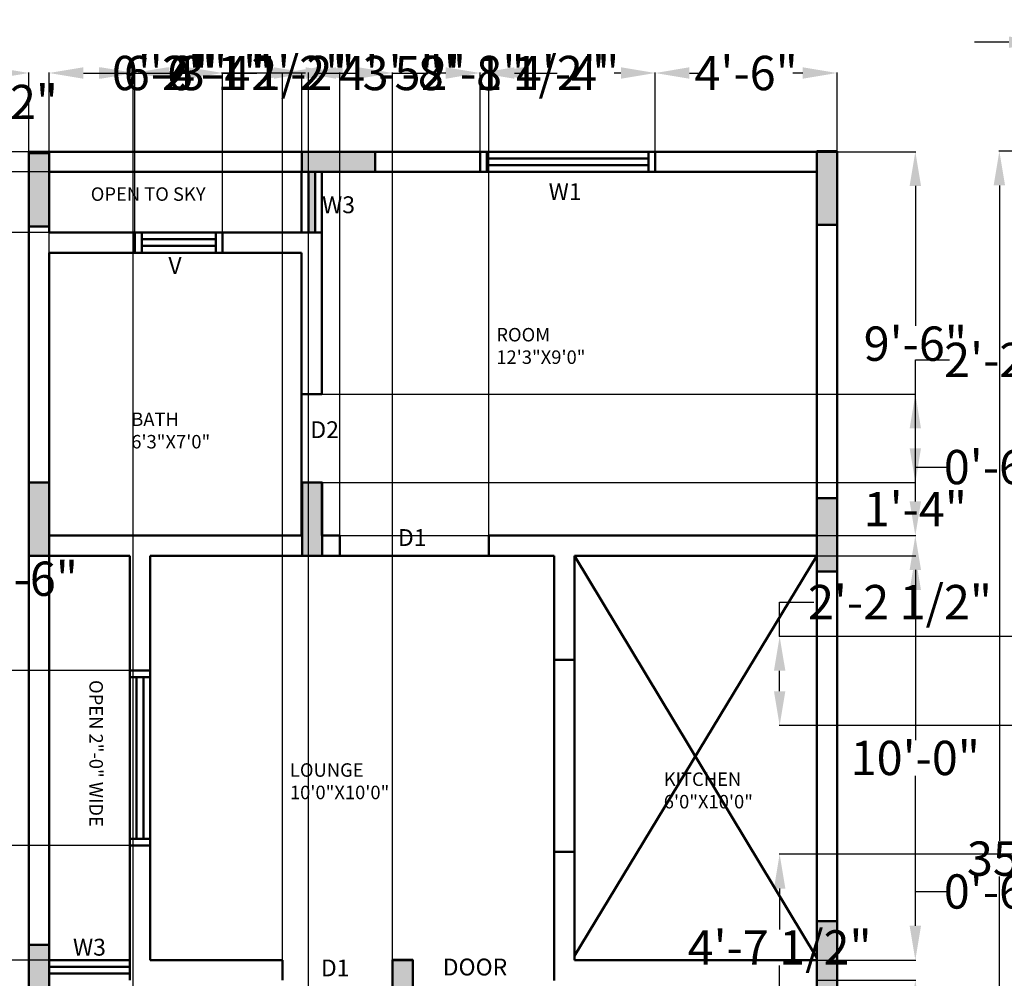
# Model space of a CAD drawing. Units: inches. Extents: x 21 to 3450, y 4 to 2137.
# Tile 4 of 14: x 2513 to 2805, y 1261 to 1546. Entities that reach past the tile are written whole.
import ezdxf

# ---------------------------------------------------------------- set-up
doc = ezdxf.new("R2010")
doc.units = ezdxf.units.IN
doc.header["$MEASUREMENT"] = 0
for name, color, linetype, lineweight in [('A-ANNO-DIMS', 2, 'Continuous', 18), ('A-ANNO-TEXT', 7, 'Continuous', 18), ('A-AREA-IDEN', 3, 'Continuous', 18), ('A-WALL', 7, 'Continuous', 50), ('A-WALL-PATT', 8, 'Continuous', 13)]:
    doc.layers.add(name, color=color, linetype=linetype, lineweight=lineweight)
doc.styles.get("Standard").update_dxf_attribs({"font": 'arial.ttf'})
doc.dimstyles.get("Standard").update_dxf_attribs({"dimtxt": 10.18, "dimasz": 10.18, "dimexe": 0.18, "dimexo": 0.0625, "dimgap": 0.09, "dimtad": 0, "dimtih": 1, "dimtoh": 1, "dimdec": 0, "dimzin": 0, "dimdsep": 46, "dimlunit": 3, "dimtxsty": 'Standard', "dimcen": 0.09, "dimadec": 0, "dimazin": 0, "dimtfac": 1, "dimtdec": 0, "dimtofl": 0, "dimtmove": 0, "dimatfit": 3, "dimfxl": 1, "dimtolj": 1, "dimtzin": 0, "dimarcsym": 0})

# ---------------------------------------------------------------- blocks, each defined once
blk = doc.blocks.new('*D8')
at = {"layer": 'A-ANNO-DIMS', "color": 0, "lineweight": -2, "transparency": 16777216}
for p, q in [((2816.85, 1506.81), (2803.73, 1506.81)), ((2803.91, 1496.63), (2803.91, 1302.07)), ((2803.91, 1096.92), (2803.91, 1291.48)), ((2999.5, 1086.74), (2803.73, 1086.74))]:
    blk.add_line(p, q, dxfattribs=at)
at = {"layer": 'A-ANNO-DIMS', "color": 0, "transparency": 16777216}
for points in [[(2802.22, 1496.63), (2805.61, 1496.63), (2803.91, 1506.81)], [(2802.22, 1096.92), (2805.61, 1096.92), (2803.91, 1086.74)]]:
    blk.add_solid(points, dxfattribs=at)
at = {"layer": 'Defpoints', "color": 0, "transparency": 16777216}
for p in [(2816.91, 1506.81), (2803.91, 1086.74), (2999.56, 1086.74)]:
    blk.add_point(p, dxfattribs=at)
at = {"layer": 'A-ANNO-DIMS', "color": 0, "transparency": 16777216, "insert": (2803.91, 1296.77), "char_height": 10.18, "attachment_point": 5}
blk.add_mtext("\\A1;35'", dxfattribs=at)
blk = doc.blocks.new('*D48')
at = {"layer": 'A-ANNO-DIMS', "color": 0, "lineweight": -2, "transparency": 16777216}
for p, q in [((2491.15, 1369.68), (2491.15, 1379.86)), ((2491.15, 1379.86), (2501.33, 1379.86)), ((2461.46, 1359.5), (2491.33, 1359.5)), ((2461.25, 1353.55), (2491.33, 1353.55)), ((2491.15, 1343.37), (2491.15, 1333.19))]:
    blk.add_line(p, q, dxfattribs=at)
at = {"layer": 'A-ANNO-DIMS', "color": 0, "transparency": 16777216}
for points in [[(2489.45, 1369.68), (2492.84, 1369.68), (2491.15, 1359.5)], [(2489.45, 1343.37), (2492.84, 1343.37), (2491.15, 1353.55)]]:
    blk.add_solid(points, dxfattribs=at)
at = {"layer": 'Defpoints', "color": 0, "transparency": 16777216}
for p in [(2461.4, 1359.5), (2491.15, 1359.5), (2461.19, 1353.55)]:
    blk.add_point(p, dxfattribs=at)
at = {"layer": 'A-ANNO-DIMS', "color": 0, "transparency": 16777216, "insert": (2514.95, 1379.86), "char_height": 10.18, "attachment_point": 5}
blk.add_mtext('\\A1;0\'-6"', dxfattribs=at)
blk = doc.blocks.new('*D63')
at = {"layer": 'A-ANNO-DIMS', "color": 0, "lineweight": -2, "transparency": 16777216}
for p, q in [((2417.71, 1189.56), (2417.71, 1521.59)), ((2427.89, 1521.41), (2451.22, 1521.41)), ((2461.4, 1189.56), (2461.4, 1521.59)), ((2461.4, 1521.41), (2471.58, 1521.41))]:
    blk.add_line(p, q, dxfattribs=at)
at = {"layer": 'A-ANNO-DIMS', "color": 0, "transparency": 16777216}
for points in [[(2427.89, 1523.11), (2427.89, 1519.72), (2417.71, 1521.41)], [(2451.22, 1523.11), (2451.22, 1519.72), (2461.4, 1521.41)]]:
    blk.add_solid(points, dxfattribs=at)
at = {"layer": 'Defpoints', "color": 0, "transparency": 16777216}
for p in [(2461.4, 1521.41), (2417.71, 1189.5), (2461.4, 1189.5)]:
    blk.add_point(p, dxfattribs=at)
at = {"layer": 'A-ANNO-DIMS', "color": 0, "transparency": 16777216, "insert": (2497.05, 1521.41), "char_height": 10.18, "attachment_point": 5}
blk.add_mtext('\\A1;3\'-7 1/2"', dxfattribs=at)
blk = doc.blocks.new('*D67')
at = {"layer": 'A-ANNO-DIMS', "color": 0, "lineweight": -2, "transparency": 16777216}
for p, q in [((2515.64, 1506.65), (2492.19, 1506.65)), ((2492.37, 1496.47), (2492.37, 1301.94)), ((2492.37, 1096.83), (2492.37, 1291.36)), ((2515.56, 1086.65), (2492.19, 1086.65))]:
    blk.add_line(p, q, dxfattribs=at)
at = {"layer": 'A-ANNO-DIMS', "color": 0, "transparency": 16777216}
for points in [[(2490.67, 1496.47), (2494.06, 1496.47), (2492.37, 1506.65)], [(2490.67, 1096.83), (2494.06, 1096.83), (2492.37, 1086.65)]]:
    blk.add_solid(points, dxfattribs=at)
at = {"layer": 'Defpoints', "color": 0, "transparency": 16777216}
for p in [(2492.37, 1506.65), (2515.71, 1506.65), (2515.62, 1086.65)]:
    blk.add_point(p, dxfattribs=at)
at = {"layer": 'A-ANNO-DIMS', "color": 0, "transparency": 16777216, "insert": (2492.37, 1296.65), "char_height": 10.18, "attachment_point": 5}
blk.add_mtext('\\A1;35\'-0"', dxfattribs=at)
blk = doc.blocks.new('*D68')
at = {"layer": 'A-ANNO-DIMS', "color": 0, "lineweight": -2, "transparency": 16777216}
for p, q in [((2505.53, 1530.01), (2495.35, 1530.01)), ((2515.71, 1506.71), (2515.71, 1530.19)), ((2521.71, 1500.71), (2521.71, 1530.19)), ((2531.89, 1530.01), (2542.07, 1530.01))]:
    blk.add_line(p, q, dxfattribs=at)
at = {"layer": 'A-ANNO-DIMS', "color": 0, "transparency": 16777216}
for points in [[(2505.53, 1531.71), (2505.53, 1528.31), (2515.71, 1530.01)], [(2531.89, 1531.71), (2531.89, 1528.31), (2521.71, 1530.01)]]:
    blk.add_solid(points, dxfattribs=at)
at = {"layer": 'Defpoints', "color": 0, "transparency": 16777216}
for p in [(2521.71, 1530.01), (2515.71, 1506.65), (2521.71, 1500.65)]:
    blk.add_point(p, dxfattribs=at)
at = {"layer": 'A-ANNO-DIMS', "color": 0, "transparency": 16777216, "insert": (2555.69, 1530.01), "char_height": 10.18, "attachment_point": 5}
blk.add_mtext('\\A1;0\'-6"', dxfattribs=at)
blk = doc.blocks.new('*D69')
at = {"layer": 'A-ANNO-DIMS', "color": 0, "lineweight": -2, "transparency": 16777216}
for p, q in [((2521.71, 1500.71), (2521.71, 1530.19)), ((2531.89, 1530.01), (2545.6, 1530.01)), ((2586.6, 1530.01), (2572.89, 1530.01)), ((2596.78, 1500.71), (2596.78, 1530.19))]:
    blk.add_line(p, q, dxfattribs=at)
at = {"layer": 'A-ANNO-DIMS', "color": 0, "transparency": 16777216}
for points in [[(2531.89, 1531.71), (2531.89, 1528.31), (2521.71, 1530.01)], [(2586.6, 1531.71), (2586.6, 1528.31), (2596.78, 1530.01)]]:
    blk.add_solid(points, dxfattribs=at)
at = {"layer": 'Defpoints', "color": 0, "transparency": 16777216}
for p in [(2596.78, 1530.01), (2521.71, 1500.65), (2596.78, 1500.65)]:
    blk.add_point(p, dxfattribs=at)
at = {"layer": 'A-ANNO-DIMS', "color": 0, "transparency": 16777216, "insert": (2559.24, 1530.01), "char_height": 10.18, "attachment_point": 5}
blk.add_mtext('\\A1;6\'-3"', dxfattribs=at)
blk = doc.blocks.new('*D70')
at = {"layer": 'A-ANNO-DIMS', "color": 0, "lineweight": -2, "transparency": 16777216}
for p, q in [((2596.78, 1500.71), (2596.78, 1530.19)), ((2606.96, 1530.01), (2609.42, 1530.01)), ((2639.52, 1530.01), (2637.07, 1530.01)), ((2649.7, 1506.71), (2649.7, 1530.19))]:
    blk.add_line(p, q, dxfattribs=at)
at = {"layer": 'A-ANNO-DIMS', "color": 0, "transparency": 16777216}
for points in [[(2606.96, 1531.71), (2606.96, 1528.31), (2596.78, 1530.01)], [(2639.52, 1531.71), (2639.52, 1528.31), (2649.7, 1530.01)]]:
    blk.add_solid(points, dxfattribs=at)
at = {"layer": 'Defpoints', "color": 0, "transparency": 16777216}
for p in [(2649.7, 1530.01), (2649.7, 1506.65), (2596.78, 1500.65)]:
    blk.add_point(p, dxfattribs=at)
at = {"layer": 'A-ANNO-DIMS', "color": 0, "transparency": 16777216, "insert": (2623.24, 1530.01), "char_height": 10.18, "attachment_point": 5}
blk.add_mtext('\\A1;4\'-5"', dxfattribs=at)
blk = doc.blocks.new('*D71')
at = {"layer": 'A-ANNO-DIMS', "color": 0, "lineweight": -2, "transparency": 16777216}
for p, q in [((2649.7, 1506.71), (2649.7, 1530.19)), ((2659.88, 1530.01), (2661.88, 1530.01)), ((2691.52, 1530.01), (2689.53, 1530.01)), ((2701.7, 1506.71), (2701.7, 1530.19))]:
    blk.add_line(p, q, dxfattribs=at)
at = {"layer": 'A-ANNO-DIMS', "color": 0, "transparency": 16777216}
for points in [[(2659.88, 1531.71), (2659.88, 1528.31), (2649.7, 1530.01)], [(2691.52, 1531.71), (2691.52, 1528.31), (2701.7, 1530.01)]]:
    blk.add_solid(points, dxfattribs=at)
at = {"layer": 'Defpoints', "color": 0, "transparency": 16777216}
for p in [(2701.7, 1530.01), (2649.7, 1506.65), (2701.7, 1506.65)]:
    blk.add_point(p, dxfattribs=at)
at = {"layer": 'A-ANNO-DIMS', "color": 0, "transparency": 16777216, "insert": (2675.7, 1530.01), "char_height": 10.18, "attachment_point": 5}
blk.add_mtext('\\A1;4\'-4"', dxfattribs=at)
blk = doc.blocks.new('*D72')
at = {"layer": 'A-ANNO-DIMS', "color": 0, "lineweight": -2, "transparency": 16777216}
for p, q in [((2701.7, 1506.71), (2701.7, 1530.19)), ((2711.88, 1530.01), (2714.88, 1530.01)), ((2745.53, 1530.01), (2742.53, 1530.01)), ((2755.71, 1506.71), (2755.71, 1530.19))]:
    blk.add_line(p, q, dxfattribs=at)
at = {"layer": 'A-ANNO-DIMS', "color": 0, "transparency": 16777216}
for points in [[(2711.88, 1531.71), (2711.88, 1528.31), (2701.7, 1530.01)], [(2745.53, 1531.71), (2745.53, 1528.31), (2755.71, 1530.01)]]:
    blk.add_solid(points, dxfattribs=at)
at = {"layer": 'Defpoints', "color": 0, "transparency": 16777216}
for p in [(2755.71, 1530.01), (2701.7, 1506.65), (2755.71, 1506.65)]:
    blk.add_point(p, dxfattribs=at)
at = {"layer": 'A-ANNO-DIMS', "color": 0, "transparency": 16777216, "insert": (2728.71, 1530.01), "char_height": 10.18, "attachment_point": 5}
blk.add_mtext('\\A1;4\'-6"', dxfattribs=at)
blk = doc.blocks.new('*D73')
at = {"layer": 'A-ANNO-DIMS', "color": 0, "lineweight": -2, "transparency": 16777216}
for p, q in [((2521.71, 1092.71), (2521.71, 1530.19)), ((2531.89, 1530.01), (2536.53, 1530.01)), ((2546.71, 1092.71), (2546.71, 1530.19)), ((2546.71, 1530.01), (2556.89, 1530.01))]:
    blk.add_line(p, q, dxfattribs=at)
at = {"layer": 'A-ANNO-DIMS', "color": 0, "transparency": 16777216}
for points in [[(2531.89, 1531.71), (2531.89, 1528.31), (2521.71, 1530.01)], [(2536.53, 1531.71), (2536.53, 1528.31), (2546.71, 1530.01)]]:
    blk.add_solid(points, dxfattribs=at)
at = {"layer": 'Defpoints', "color": 0, "transparency": 16777216}
for p in [(2546.71, 1530.01), (2521.71, 1092.65), (2546.71, 1092.65)]:
    blk.add_point(p, dxfattribs=at)
at = {"layer": 'A-ANNO-DIMS', "color": 0, "transparency": 16777216, "insert": (2570.59, 1530.01), "char_height": 10.18, "attachment_point": 5}
blk.add_mtext('\\A1;2\'-1"', dxfattribs=at)
blk = doc.blocks.new('*D74')
at = {"layer": 'A-ANNO-DIMS', "color": 0, "lineweight": -2, "transparency": 16777216}
for p, q in [((2546.71, 1092.71), (2546.71, 1530.19)), ((2556.89, 1530.01), (2558.88, 1530.01)), ((2588.53, 1530.01), (2586.53, 1530.01)), ((2598.71, 1092.71), (2598.71, 1530.19))]:
    blk.add_line(p, q, dxfattribs=at)
at = {"layer": 'A-ANNO-DIMS', "color": 0, "transparency": 16777216}
for points in [[(2556.89, 1531.71), (2556.89, 1528.31), (2546.71, 1530.01)], [(2588.53, 1531.71), (2588.53, 1528.31), (2598.71, 1530.01)]]:
    blk.add_solid(points, dxfattribs=at)
at = {"layer": 'Defpoints', "color": 0, "transparency": 16777216}
for p in [(2598.71, 1530.01), (2546.71, 1092.65), (2598.71, 1092.65)]:
    blk.add_point(p, dxfattribs=at)
at = {"layer": 'A-ANNO-DIMS', "color": 0, "transparency": 16777216, "insert": (2572.71, 1530.01), "char_height": 10.18, "attachment_point": 5}
blk.add_mtext('\\A1;4\'-4"', dxfattribs=at)
blk = doc.blocks.new('*D75')
at = {"layer": 'A-ANNO-DIMS', "color": 0, "lineweight": -2, "transparency": 16777216}
for p, q in [((2598.71, 1092.71), (2598.71, 1530.19)), ((2608.89, 1530.01), (2613.53, 1530.01)), ((2623.71, 1092.71), (2623.71, 1530.19)), ((2623.71, 1530.01), (2633.89, 1530.01))]:
    blk.add_line(p, q, dxfattribs=at)
at = {"layer": 'A-ANNO-DIMS', "color": 0, "transparency": 16777216}
for points in [[(2608.89, 1531.71), (2608.89, 1528.31), (2598.71, 1530.01)], [(2613.53, 1531.71), (2613.53, 1528.31), (2623.71, 1530.01)]]:
    blk.add_solid(points, dxfattribs=at)
at = {"layer": 'Defpoints', "color": 0, "transparency": 16777216}
for p in [(2623.71, 1530.01), (2598.71, 1092.65), (2623.71, 1092.65)]:
    blk.add_point(p, dxfattribs=at)
at = {"layer": 'A-ANNO-DIMS', "color": 0, "transparency": 16777216, "insert": (2647.59, 1530.01), "char_height": 10.18, "attachment_point": 5}
blk.add_mtext('\\A1;2\'-1"', dxfattribs=at)
blk = doc.blocks.new('*D77')
at = {"layer": 'A-ANNO-DIMS', "color": 0, "lineweight": -2, "transparency": 16777216}
for p, q in [((2778.96, 1276.83), (2778.96, 1287.01)), ((2778.96, 1287.01), (2789.14, 1287.01)), ((2749.77, 1266.65), (2779.14, 1266.65)), ((2749.77, 1260.65), (2779.14, 1260.65)), ((2778.96, 1250.47), (2778.96, 1240.29))]:
    blk.add_line(p, q, dxfattribs=at)
at = {"layer": 'A-ANNO-DIMS', "color": 0, "transparency": 16777216}
for points in [[(2777.26, 1276.83), (2780.65, 1276.83), (2778.96, 1266.65)], [(2777.26, 1250.47), (2780.65, 1250.47), (2778.96, 1260.65)]]:
    blk.add_solid(points, dxfattribs=at)
at = {"layer": 'Defpoints', "color": 0, "transparency": 16777216}
for p in [(2749.71, 1266.65), (2778.96, 1266.65), (2749.71, 1260.65)]:
    blk.add_point(p, dxfattribs=at)
at = {"layer": 'A-ANNO-DIMS', "color": 0, "transparency": 16777216, "insert": (2802.76, 1287.01), "char_height": 10.18, "attachment_point": 5}
blk.add_mtext('\\A1;0\'-6"', dxfattribs=at)
blk = doc.blocks.new('*D78')
at = {"layer": 'A-ANNO-DIMS', "color": 0, "lineweight": -2, "transparency": 16777216}
for p, q in [((2749.77, 1386.65), (2779.14, 1386.65)), ((2778.96, 1376.47), (2778.96, 1331.94)), ((2778.96, 1276.83), (2778.96, 1321.36)), ((2749.77, 1266.65), (2779.14, 1266.65))]:
    blk.add_line(p, q, dxfattribs=at)
at = {"layer": 'A-ANNO-DIMS', "color": 0, "transparency": 16777216}
for points in [[(2777.26, 1376.47), (2780.65, 1376.47), (2778.96, 1386.65)], [(2777.26, 1276.83), (2780.65, 1276.83), (2778.96, 1266.65)]]:
    blk.add_solid(points, dxfattribs=at)
at = {"layer": 'Defpoints', "color": 0, "transparency": 16777216}
for p in [(2749.71, 1386.65), (2778.96, 1386.65), (2749.71, 1266.65)]:
    blk.add_point(p, dxfattribs=at)
at = {"layer": 'A-ANNO-DIMS', "color": 0, "transparency": 16777216, "insert": (2778.96, 1326.65), "char_height": 10.18, "attachment_point": 5}
blk.add_mtext('\\A1;10\'-0"', dxfattribs=at)
blk = doc.blocks.new('*D79')
at = {"layer": 'A-ANNO-DIMS', "color": 0, "lineweight": -2, "transparency": 16777216}
for p, q in [((2778.96, 1402.83), (2778.96, 1413.01)), ((2778.96, 1413.01), (2789.14, 1413.01)), ((2749.77, 1392.65), (2779.14, 1392.65)), ((2749.77, 1386.65), (2779.14, 1386.65)), ((2778.96, 1376.47), (2778.96, 1366.29))]:
    blk.add_line(p, q, dxfattribs=at)
at = {"layer": 'A-ANNO-DIMS', "color": 0, "transparency": 16777216}
for points in [[(2777.26, 1402.83), (2780.65, 1402.83), (2778.96, 1392.65)], [(2777.26, 1376.47), (2780.65, 1376.47), (2778.96, 1386.65)]]:
    blk.add_solid(points, dxfattribs=at)
at = {"layer": 'Defpoints', "color": 0, "transparency": 16777216}
for p in [(2749.71, 1392.65), (2778.96, 1392.65), (2749.71, 1386.65)]:
    blk.add_point(p, dxfattribs=at)
at = {"layer": 'A-ANNO-DIMS', "color": 0, "transparency": 16777216, "insert": (2802.76, 1413.01), "char_height": 10.18, "attachment_point": 5}
blk.add_mtext('\\A1;0\'-6"', dxfattribs=at)
blk = doc.blocks.new('*D80')
at = {"layer": 'A-ANNO-DIMS', "color": 0, "lineweight": -2, "transparency": 16777216}
for p, q in [((2755.77, 1506.65), (2779.14, 1506.65)), ((2778.96, 1496.47), (2778.96, 1454.94)), ((2778.96, 1402.83), (2778.96, 1444.36)), ((2749.77, 1392.65), (2779.14, 1392.65))]:
    blk.add_line(p, q, dxfattribs=at)
at = {"layer": 'A-ANNO-DIMS', "color": 0, "transparency": 16777216}
for points in [[(2777.26, 1496.47), (2780.65, 1496.47), (2778.96, 1506.65)], [(2777.26, 1402.83), (2780.65, 1402.83), (2778.96, 1392.65)]]:
    blk.add_solid(points, dxfattribs=at)
at = {"layer": 'Defpoints', "color": 0, "transparency": 16777216}
for p in [(2755.71, 1506.65), (2778.96, 1506.65), (2749.71, 1392.65)]:
    blk.add_point(p, dxfattribs=at)
at = {"layer": 'A-ANNO-DIMS', "color": 0, "transparency": 16777216, "insert": (2778.96, 1449.65), "char_height": 10.18, "attachment_point": 5}
blk.add_mtext('\\A1;9\'-6"', dxfattribs=at)
blk = doc.blocks.new('*D81')
at = {"layer": 'A-ANNO-DIMS', "color": 0, "lineweight": -2, "transparency": 16777216}
for p, q in [((2492.37, 1510.83), (2492.37, 1521.01)), ((2521.64, 1500.65), (2492.19, 1500.65)), ((2521.64, 1482.65), (2492.19, 1482.65)), ((2492.37, 1472.47), (2492.37, 1462.29))]:
    blk.add_line(p, q, dxfattribs=at)
at = {"layer": 'A-ANNO-DIMS', "color": 0, "transparency": 16777216}
for points in [[(2490.67, 1510.83), (2494.06, 1510.83), (2492.37, 1500.65)], [(2490.67, 1472.47), (2494.06, 1472.47), (2492.37, 1482.65)]]:
    blk.add_solid(points, dxfattribs=at)
at = {"layer": 'Defpoints', "color": 0, "transparency": 16777216}
for p in [(2492.37, 1500.65), (2521.71, 1500.65), (2521.71, 1482.65)]:
    blk.add_point(p, dxfattribs=at)
at = {"layer": 'A-ANNO-DIMS', "color": 0, "transparency": 16777216, "insert": (2492.37, 1491.65), "char_height": 10.18, "attachment_point": 5}
blk.add_mtext('\\A1;1\'-6"', dxfattribs=at)
blk = doc.blocks.new('*D82')
at = {"layer": 'A-ANNO-DIMS', "color": 0, "lineweight": -2, "transparency": 16777216}
for p, q in [((2778.96, 1434.65), (2778.96, 1444.83)), ((2778.96, 1444.83), (2789.14, 1444.83)), ((2602.77, 1434.65), (2779.14, 1434.65)), ((2778.96, 1418.61), (2778.96, 1424.47)), ((2602.9, 1408.43), (2779.14, 1408.43))]:
    blk.add_line(p, q, dxfattribs=at)
at = {"layer": 'A-ANNO-DIMS', "color": 0, "transparency": 16777216}
for points in [[(2777.26, 1424.47), (2780.65, 1424.47), (2778.96, 1434.65)], [(2777.26, 1418.61), (2780.65, 1418.61), (2778.96, 1408.43)]]:
    blk.add_solid(points, dxfattribs=at)
at = {"layer": 'Defpoints', "color": 0, "transparency": 16777216}
for p in [(2602.71, 1434.65), (2778.96, 1434.65), (2602.84, 1408.43)]:
    blk.add_point(p, dxfattribs=at)
at = {"layer": 'A-ANNO-DIMS', "color": 0, "transparency": 16777216, "insert": (2802.84, 1444.83), "char_height": 10.18, "attachment_point": 5}
blk.add_mtext('\\A1;2\'-2"', dxfattribs=at)
blk = doc.blocks.new('*D83')
at = {"layer": 'A-ANNO-DIMS', "color": 0, "lineweight": -2, "transparency": 16777216}
for p, q in [((2778.96, 1418.61), (2778.96, 1428.79)), ((2602.9, 1408.43), (2779.14, 1408.43)), ((2602.77, 1392.65), (2779.14, 1392.65)), ((2778.96, 1382.47), (2778.96, 1372.29))]:
    blk.add_line(p, q, dxfattribs=at)
at = {"layer": 'A-ANNO-DIMS', "color": 0, "transparency": 16777216}
for points in [[(2777.26, 1418.61), (2780.65, 1418.61), (2778.96, 1408.43)], [(2777.26, 1382.47), (2780.65, 1382.47), (2778.96, 1392.65)]]:
    blk.add_solid(points, dxfattribs=at)
at = {"layer": 'Defpoints', "color": 0, "transparency": 16777216}
for p in [(2602.84, 1408.43), (2778.96, 1408.43), (2602.71, 1392.65)]:
    blk.add_point(p, dxfattribs=at)
at = {"layer": 'A-ANNO-DIMS', "color": 0, "transparency": 16777216, "insert": (2778.96, 1400.54), "char_height": 10.18, "attachment_point": 5}
blk.add_mtext('\\A1;1\'-4"', dxfattribs=at)
blk = doc.blocks.new('*D84')
at = {"layer": 'A-ANNO-DIMS', "color": 0, "lineweight": -2, "transparency": 16777216}
for p, q in [((2597.89, 1530.01), (2587.71, 1530.01)), ((2608.07, 1392.71), (2608.07, 1530.19)), ((2652.26, 1392.71), (2652.26, 1530.19)), ((2662.44, 1530.01), (2672.62, 1530.01))]:
    blk.add_line(p, q, dxfattribs=at)
at = {"layer": 'A-ANNO-DIMS', "color": 0, "transparency": 16777216}
for points in [[(2597.89, 1531.71), (2597.89, 1528.31), (2608.07, 1530.01)], [(2662.44, 1531.71), (2662.44, 1528.31), (2652.26, 1530.01)]]:
    blk.add_solid(points, dxfattribs=at)
at = {"layer": 'Defpoints', "color": 0, "transparency": 16777216}
for p in [(2652.26, 1530.01), (2608.07, 1392.65), (2652.26, 1392.65)]:
    blk.add_point(p, dxfattribs=at)
at = {"layer": 'A-ANNO-DIMS', "color": 0, "transparency": 16777216, "insert": (2630.16, 1530.01), "char_height": 10.18, "attachment_point": 5}
blk.add_mtext('\\A1;3\'-8"', dxfattribs=at)
blk = doc.blocks.new('*D85')
at = {"layer": 'A-ANNO-DIMS', "color": 0, "lineweight": -2, "transparency": 16777216}
for p, q in [((2591.07, 1266.71), (2591.07, 1530.19)), ((2601.25, 1530.01), (2613.53, 1530.01)), ((2623.71, 1266.71), (2623.71, 1530.19)), ((2623.71, 1530.01), (2633.89, 1530.01))]:
    blk.add_line(p, q, dxfattribs=at)
at = {"layer": 'A-ANNO-DIMS', "color": 0, "transparency": 16777216}
for points in [[(2601.25, 1531.71), (2601.25, 1528.31), (2591.07, 1530.01)], [(2613.53, 1531.71), (2613.53, 1528.31), (2623.71, 1530.01)]]:
    blk.add_solid(points, dxfattribs=at)
at = {"layer": 'Defpoints', "color": 0, "transparency": 16777216}
for p in [(2623.71, 1530.01), (2591.07, 1266.65), (2623.71, 1266.65)]:
    blk.add_point(p, dxfattribs=at)
at = {"layer": 'A-ANNO-DIMS', "color": 0, "transparency": 16777216, "insert": (2659.45, 1530.01), "char_height": 10.18, "attachment_point": 5}
blk.add_mtext('\\A1;2\'-8 1/2"', dxfattribs=at)
blk = doc.blocks.new('*D89')
at = {"layer": 'A-ANNO-DIMS', "color": 0, "lineweight": -2, "transparency": 16777216}
for p, q in [((2545.64, 1352.65), (2492.19, 1352.65)), ((2492.37, 1342.47), (2492.37, 1331.83)), ((2492.37, 1310.83), (2492.37, 1321.47)), ((2545.64, 1300.65), (2492.19, 1300.65))]:
    blk.add_line(p, q, dxfattribs=at)
at = {"layer": 'A-ANNO-DIMS', "color": 0, "transparency": 16777216}
for points in [[(2490.67, 1342.47), (2494.06, 1342.47), (2492.37, 1352.65)], [(2490.67, 1310.83), (2494.06, 1310.83), (2492.37, 1300.65)]]:
    blk.add_solid(points, dxfattribs=at)
at = {"layer": 'Defpoints', "color": 0, "transparency": 16777216}
for p in [(2492.37, 1352.65), (2545.71, 1352.65), (2545.71, 1300.65)]:
    blk.add_point(p, dxfattribs=at)
at = {"layer": 'A-ANNO-DIMS', "color": 0, "transparency": 16777216, "insert": (2492.37, 1326.65), "char_height": 10.18, "attachment_point": 5}
blk.add_mtext('\\A1;4\'-4"', dxfattribs=at)
blk = doc.blocks.new('*D90')
at = {"layer": 'A-ANNO-DIMS', "color": 0, "lineweight": -2, "transparency": 16777216}
for p, q in [((2545.64, 1300.65), (2492.19, 1300.65)), ((2492.37, 1290.47), (2492.37, 1288.94)), ((2492.37, 1276.83), (2492.37, 1278.36)), ((2545.64, 1266.65), (2492.19, 1266.65))]:
    blk.add_line(p, q, dxfattribs=at)
at = {"layer": 'A-ANNO-DIMS', "color": 0, "transparency": 16777216}
for points in [[(2490.67, 1290.47), (2494.06, 1290.47), (2492.37, 1300.65)], [(2490.67, 1276.83), (2494.06, 1276.83), (2492.37, 1266.65)]]:
    blk.add_solid(points, dxfattribs=at)
at = {"layer": 'Defpoints', "color": 0, "transparency": 16777216}
for p in [(2492.37, 1300.65), (2545.71, 1300.65), (2545.71, 1266.65)]:
    blk.add_point(p, dxfattribs=at)
at = {"layer": 'A-ANNO-DIMS', "color": 0, "transparency": 16777216, "insert": (2492.37, 1283.65), "char_height": 10.18, "attachment_point": 5}
blk.add_mtext('\\A1;2\'-10"', dxfattribs=at)
blk = doc.blocks.new('*D91')
at = {"layer": 'A-ANNO-DIMS', "color": 0, "lineweight": -2, "transparency": 16777216}
for p, q in [((2521.71, 1476.71), (2521.71, 1530.19)), ((2531.89, 1530.01), (2537.03, 1530.01)), ((2547.21, 1476.71), (2547.21, 1530.19)), ((2547.21, 1530.01), (2557.39, 1530.01))]:
    blk.add_line(p, q, dxfattribs=at)
at = {"layer": 'A-ANNO-DIMS', "color": 0, "transparency": 16777216}
for points in [[(2531.89, 1531.71), (2531.89, 1528.31), (2521.71, 1530.01)], [(2537.03, 1531.71), (2537.03, 1528.31), (2547.21, 1530.01)]]:
    blk.add_solid(points, dxfattribs=at)
at = {"layer": 'Defpoints', "color": 0, "transparency": 16777216}
for p in [(2547.21, 1530.01), (2521.71, 1476.65), (2547.21, 1476.65)]:
    blk.add_point(p, dxfattribs=at)
at = {"layer": 'A-ANNO-DIMS', "color": 0, "transparency": 16777216, "insert": (2582.95, 1530.01), "char_height": 10.18, "attachment_point": 5}
blk.add_mtext('\\A1;2\'-1 1/2"', dxfattribs=at)
blk = doc.blocks.new('*D92')
at = {"layer": 'A-ANNO-DIMS', "color": 0, "lineweight": -2, "transparency": 16777216}
for p, q in [((2547.21, 1476.71), (2547.21, 1530.19)), ((2557.39, 1530.01), (2563.03, 1530.01)), ((2573.21, 1476.71), (2573.21, 1530.19)), ((2573.21, 1530.01), (2583.39, 1530.01))]:
    blk.add_line(p, q, dxfattribs=at)
at = {"layer": 'A-ANNO-DIMS', "color": 0, "transparency": 16777216}
for points in [[(2557.39, 1531.71), (2557.39, 1528.31), (2547.21, 1530.01)], [(2563.03, 1531.71), (2563.03, 1528.31), (2573.21, 1530.01)]]:
    blk.add_solid(points, dxfattribs=at)
at = {"layer": 'Defpoints', "color": 0, "transparency": 16777216}
for p in [(2573.21, 1530.01), (2547.21, 1476.65), (2573.21, 1476.65)]:
    blk.add_point(p, dxfattribs=at)
at = {"layer": 'A-ANNO-DIMS', "color": 0, "transparency": 16777216, "insert": (2597.09, 1530.01), "char_height": 10.18, "attachment_point": 5}
blk.add_mtext('\\A1;2\'-2"', dxfattribs=at)
blk = doc.blocks.new('*D96')
at = {"layer": 'A-ANNO-DIMS', "color": 0, "lineweight": -2, "transparency": 16777216}
for p, q in [((2806.73, 1539.16), (2796.55, 1539.16)), ((2816.91, 1506.81), (2816.91, 1539.34)), ((2822.91, 1500.81), (2822.91, 1539.34)), ((2833.09, 1539.16), (2843.27, 1539.16))]:
    blk.add_line(p, q, dxfattribs=at)
at = {"layer": 'A-ANNO-DIMS', "color": 0, "transparency": 16777216}
for points in [[(2806.73, 1540.85), (2806.73, 1537.46), (2816.91, 1539.16)], [(2833.09, 1540.85), (2833.09, 1537.46), (2822.91, 1539.16)]]:
    blk.add_solid(points, dxfattribs=at)
at = {"layer": 'Defpoints', "color": 0, "transparency": 16777216}
for p in [(2822.91, 1539.16), (2816.91, 1506.74), (2822.91, 1500.74)]:
    blk.add_point(p, dxfattribs=at)
at = {"layer": 'A-ANNO-DIMS', "color": 0, "transparency": 16777216, "insert": (2856.89, 1539.16), "char_height": 10.18, "attachment_point": 5}
blk.add_mtext('\\A1;0\'-6"', dxfattribs=at)
blk = doc.blocks.new('*D119')
at = {"layer": 'A-ANNO-DIMS', "color": 0, "lineweight": -2, "transparency": 16777216}
for p, q in [((2738.66, 1362.74), (2738.66, 1372.92)), ((2738.66, 1372.92), (2748.84, 1372.92)), ((2972.85, 1362.74), (2738.48, 1362.74)), ((2738.66, 1346.47), (2738.66, 1352.56)), ((2972.85, 1336.29), (2738.48, 1336.29))]:
    blk.add_line(p, q, dxfattribs=at)
at = {"layer": 'A-ANNO-DIMS', "color": 0, "transparency": 16777216}
for points in [[(2736.97, 1352.56), (2740.36, 1352.56), (2738.66, 1362.74)], [(2736.97, 1346.47), (2740.36, 1346.47), (2738.66, 1336.29)]]:
    blk.add_solid(points, dxfattribs=at)
at = {"layer": 'Defpoints', "color": 0, "transparency": 16777216}
for p in [(2738.66, 1362.74), (2972.91, 1362.74), (2972.91, 1336.29)]:
    blk.add_point(p, dxfattribs=at)
at = {"layer": 'A-ANNO-DIMS', "color": 0, "transparency": 16777216, "insert": (2774.41, 1372.92), "char_height": 10.18, "attachment_point": 5}
blk.add_mtext('\\A1;2\'-2 1/2"', dxfattribs=at)
blk = doc.blocks.new('*D120')
at = {"layer": 'A-ANNO-DIMS', "color": 0, "lineweight": -2, "transparency": 16777216}
for p, q in [((2972.85, 1298.07), (2738.48, 1298.07)), ((2738.66, 1287.89), (2738.66, 1275.76)), ((2738.66, 1252.92), (2738.66, 1265.05)), ((2972.85, 1242.74), (2738.48, 1242.74))]:
    blk.add_line(p, q, dxfattribs=at)
at = {"layer": 'A-ANNO-DIMS', "color": 0, "transparency": 16777216}
for points in [[(2736.97, 1287.89), (2740.36, 1287.89), (2738.66, 1298.07)], [(2736.97, 1252.92), (2740.36, 1252.92), (2738.66, 1242.74)]]:
    blk.add_solid(points, dxfattribs=at)
at = {"layer": 'Defpoints', "color": 0, "transparency": 16777216}
for p in [(2738.66, 1298.07), (2972.91, 1298.07), (2972.91, 1242.74)]:
    blk.add_point(p, dxfattribs=at)
at = {"layer": 'A-ANNO-DIMS', "color": 0, "transparency": 16777216, "insert": (2738.66, 1270.41), "char_height": 10.18, "attachment_point": 5}
blk.add_mtext('\\A1;4\'-7 1/2"', dxfattribs=at)

msp = doc.modelspace()

# ---------------------------------------------------------------- hatches: boundary and pattern name
at = {"layer": 'A-WALL-PATT'}
h = msp.add_hatch(color=256, dxfattribs=at)
h.dxf.hatch_style = 1
h.paths.add_polyline_path([(2521.71, 1506.22), (2515.71, 1506.22), (2515.71, 1484.44), (2521.71, 1484.44)])
h.paths.add_polyline_path([(2618.57, 1506.65), (2596.78, 1506.65), (2596.78, 1500.65), (2618.57, 1500.65)])
h.paths.add_polyline_path([(2755.71, 1506.65), (2749.71, 1506.65), (2749.71, 1484.98), (2755.71, 1484.98)])
h.paths.add_polyline_path([(2755.71, 1403.77), (2749.71, 1403.77), (2749.71, 1381.98), (2755.71, 1381.98)])
h.paths.add_polyline_path([(2602.71, 1408.43), (2596.84, 1408.43), (2596.84, 1386.65), (2602.84, 1386.65), (2602.84, 1392.65), (2602.71, 1392.65)])
h.paths.add_polyline_path([(2755.71, 1278.18), (2749.71, 1278.18), (2749.71, 1256.4), (2755.71, 1256.4)])
h.paths.add_polyline_path([(2521.71, 1271.12), (2515.71, 1271.12), (2515.71, 1249.33), (2521.71, 1249.33)])
h.paths.add_polyline_path([(2521.71, 1408.43), (2515.71, 1408.43), (2515.71, 1386.65), (2521.71, 1386.65)])
h.paths.add_polyline_path([(2629.71, 1266.65), (2623.71, 1266.65), (2623.71, 1244.92), (2629.71, 1244.92)])
h.paths.add_polyline_path([(2521.62, 1108.43), (2515.71, 1108.43), (2515.71, 1086.65), (2521.62, 1086.65)])
h.paths.add_polyline_path([(2629.43, 1108.43), (2623.71, 1108.43), (2623.71, 1092.65), (2623.43, 1086.65), (2629.43, 1086.65)])
h.paths.add_polyline_path([(2755.71, 1108.43), (2749.71, 1108.43), (2749.71, 1086.65), (2755.71, 1086.65)])
h = msp.add_hatch(color=256, dxfattribs=at)
h.dxf.hatch_style = 1
h.paths.add_polyline_path([(2600.71, 1500.65), (2598.71, 1500.65), (2598.71, 1482.65), (2600.71, 1482.65)])

# ---------------------------------------------------------------- linework, layer by layer
at = {"layer": 'A-WALL'}
for p, q in [((2515.71, 1086.65), (2515.71, 1506.65)), ((2515.71, 1506.65), (2755.71, 1506.65)), ((2649.7, 1500.65), (2649.7, 1506.65)), ((2651.7, 1500.65), (2651.7, 1506.65)), ((2699.7, 1500.65), (2699.7, 1506.65)), ((2701.7, 1500.65), (2701.7, 1506.65)), ((2755.71, 1506.65), (2755.71, 1086.65)), ((2651.7, 1504.65), (2699.7, 1504.65)), ((2521.71, 1500.65), (2749.71, 1500.65)), ((2521.71, 1482.65), (2521.71, 1500.65)), ((2596.71, 1500.65), (2596.71, 1482.65)), ((2598.71, 1482.65), (2598.71, 1500.65)), ((2600.71, 1482.65), (2600.71, 1500.65)), ((2602.71, 1500.65), (2602.71, 1434.65)), ((2651.7, 1502.65), (2699.7, 1502.65)), ((2749.71, 1500.65), (2749.71, 1392.65)), ((2521.71, 1482.65), (2596.71, 1482.65)), ((2547.21, 1482.65), (2547.21, 1476.65)), ((2549.21, 1482.65), (2549.21, 1476.65)), ((2571.21, 1482.65), (2571.21, 1476.65)), ((2573.21, 1482.65), (2573.21, 1476.65)), ((2596.71, 1482.65), (2602.71, 1482.65)), ((2549.21, 1480.65), (2571.21, 1480.65)), ((2521.71, 1476.65), (2596.71, 1476.65)), ((2521.71, 1392.65), (2521.71, 1476.65)), ((2549.21, 1478.65), (2571.21, 1478.65)), ((2596.71, 1476.65), (2596.71, 1392.65)), ((2596.71, 1434.65), (2602.71, 1434.65)), ((2602.71, 1408.43), (2602.71, 1392.65)), ((2521.71, 1392.65), (2596.71, 1392.65)), ((2602.71, 1392.65), (2608.07, 1392.65)), ((2608.07, 1392.65), (2608.07, 1386.65)), ((2652.26, 1386.65), (2652.26, 1392.65)), ((2652.26, 1392.65), (2749.71, 1392.65)), ((2521.71, 1386.65), (2545.71, 1386.65)), ((2521.71, 1266.65), (2521.71, 1386.65)), ((2545.71, 1386.65), (2545.71, 1266.65)), ((2551.71, 1386.65), (2551.71, 1266.65)), ((2551.71, 1386.65), (2671.71, 1386.65)), ((2671.71, 1386.65), (2671.71, 1266.65)), ((2677.71, 1386.65), (2677.71, 1266.65)), ((2677.71, 1386.65), (2749.71, 1386.65)), ((2677.71, 1386.65), (2749.71, 1267.29)), ((2749.71, 1386.65), (2677.71, 1267.94)), ((2749.71, 1386.65), (2749.71, 1266.65)), ((2671.71, 1355.74), (2677.71, 1355.74)), ((2551.71, 1352.65), (2545.71, 1352.65)), ((2551.71, 1350.65), (2545.71, 1350.65)), ((2547.71, 1350.65), (2547.71, 1302.65)), ((2549.71, 1350.65), (2549.71, 1302.65)), ((2549.71, 1350.65), (2549.71, 1302.65)), ((2551.71, 1302.65), (2545.71, 1302.65)), ((2551.71, 1300.65), (2545.71, 1300.65)), ((2671.71, 1298.78), (2677.71, 1298.78)), ((2521.71, 1266.65), (2545.71, 1266.65)), ((2521.71, 1266.65), (2521.71, 1260.65)), ((2545.71, 1266.65), (2545.71, 1260.65)), ((2551.71, 1266.65), (2591.07, 1266.65)), ((2591.07, 1266.65), (2591.07, 1260.65)), ((2623.71, 1266.65), (2629.71, 1266.65)), ((2671.71, 1266.65), (2671.71, 1260.57)), ((2677.71, 1266.65), (2749.71, 1266.65)), ((2545.71, 1264.65), (2521.71, 1264.65)), ((2545.71, 1262.65), (2521.71, 1262.65))]:
    msp.add_line(p, q, dxfattribs=at)
for points in [[(2515.71, 1506.22), (2521.71, 1506.22), (2521.71, 1484.44), (2515.71, 1484.44)], [(2596.78, 1500.65), (2596.78, 1506.65), (2618.57, 1506.65), (2618.57, 1500.65)], [(2749.71, 1506.76), (2755.71, 1506.76), (2755.71, 1484.98), (2749.71, 1484.98)], [(2515.71, 1408.43), (2521.71, 1408.43), (2521.71, 1386.65), (2515.71, 1386.65)], [(2596.84, 1408.43), (2602.84, 1408.43), (2602.84, 1386.65), (2596.84, 1386.65)], [(2749.71, 1403.77), (2755.71, 1403.77), (2755.71, 1381.98), (2749.71, 1381.98)], [(2749.71, 1278.18), (2755.71, 1278.18), (2755.71, 1256.4), (2749.71, 1256.4)], [(2515.71, 1271.12), (2521.71, 1271.12), (2521.71, 1249.33), (2515.71, 1249.33)], [(2623.71, 1266.7), (2629.71, 1266.7), (2629.71, 1244.92), (2623.71, 1244.92)]]:
    msp.add_lwpolyline(points, close=True, dxfattribs=at)

# ---------------------------------------------------------------- texts
at = {"layer": 'A-ANNO-TEXT', "attachment_point": 1}
for s, width, insert, char_height in [('W1', 12.1398, (2670.07, 1497.29), 5), ('OPEN TO SKY', 50.8458, (2534.08, 1496.06), 4), ('W3', 12.1398, (2602.78, 1493.39), 5), ('V', 12.1398, (2557.14, 1475.37), 5), ('D2', 12.1398, (2599.3, 1426.61), 5), ('D1', 12.1398, (2625.32, 1394.59), 5), ('W3', 12.1398, (2528.81, 1272.96), 5), ('D1', 12.1398, (2602.43, 1266.81), 5), ('DOOR', 12.1398, (2638.61, 1267.08), 5)]:
    msp.add_mtext_dynamic_manual_height_columns(s, width=width, gutter_width=1, heights=[0], dxfattribs=dict(at, insert=insert, char_height=char_height))
at = {"layer": 'A-ANNO-TEXT', "insert": (2537.68, 1349.79), "char_height": 4, "attachment_point": 1, "rotation": 270}
msp.add_mtext_dynamic_manual_height_columns('OPEN 2"-0" WIDE', width=50.8458, gutter_width=1, heights=[0], dxfattribs=at)
at = {"layer": 'A-AREA-IDEN', "char_height": 4, "attachment_point": 1}
for s, insert in [('ROOM\\P12\'3"X9\'0"', (2654.52, 1454.31)), ('BATH\\P6\'3"X7\'0"', (2546.11, 1429.21)), ('LOUNGE\\P10\'0"X10\'0"', (2593.23, 1325.07)), ('KITCHEN\\P6\'0"X10\'0"', (2704.25, 1322.34))]:
    msp.add_mtext_dynamic_manual_height_columns(s, width=50.8458, gutter_width=1, heights=[0], dxfattribs=dict(at, insert=insert))

# ---------------------------------------------------------------- dimensions: what is measured, and where the dimension line sits
at = {"layer": 'A-ANNO-DIMS'}
for base, p1, p2, picture, middle in [((2547.21, 1530.01), (2521.71, 1476.65), (2547.21, 1476.65), '*D91', (2582.95, 1530.01)), ((2623.71, 1530.01), (2591.07, 1266.65), (2623.71, 1266.65), '*D85', (2659.45, 1530.01)), ((2822.91, 1539.16), (2816.91, 1506.74), (2822.91, 1500.74), '*D96', (2856.89, 1539.16)), ((2461.4, 1521.41), (2417.71, 1189.5), (2461.4, 1189.5), '*D63', (2497.05, 1521.41)), ((2521.71, 1530.01), (2515.71, 1506.65), (2521.71, 1500.65), '*D68', (2555.69, 1530.01)), ((2596.78, 1530.01), (2521.71, 1500.65), (2596.78, 1500.65), '*D69', (2559.24, 1530.01)), ((2546.71, 1530.01), (2521.71, 1092.65), (2546.71, 1092.65), '*D73', (2570.59, 1530.01)), ((2598.71, 1530.01), (2546.71, 1092.65), (2598.71, 1092.65), '*D74', (2572.71, 1530.01)), ((2573.21, 1530.01), (2547.21, 1476.65), (2573.21, 1476.65), '*D92', (2597.09, 1530.01)), ((2652.26, 1530.01), (2608.07, 1392.65), (2652.26, 1392.65), '*D84', (2630.16, 1530.01)), ((2649.7, 1530.01), (2596.78, 1500.65), (2649.7, 1506.65), '*D70', (2623.24, 1530.01)), ((2623.71, 1530.01), (2598.71, 1092.65), (2623.71, 1092.65), '*D75', (2647.59, 1530.01)), ((2701.7, 1530.01), (2649.7, 1506.65), (2701.7, 1506.65), '*D71', (2675.7, 1530.01)), ((2755.71, 1530.01), (2701.7, 1506.65), (2755.71, 1506.65), '*D72', (2728.71, 1530.01))]:
    dim = msp.add_linear_dim(base=base, p1=p1, p2=p2, dimstyle='Standard', override={"dimdec": 1, "dimlfac": 1, "dimrnd": 0, "dimzin": 1, "dimdsep": 46, "dimlunit": 4, "dimfrac": 2}, dxfattribs=at)
    dim.commit()
    dim.dimension.update_dxf_attribs({"geometry": picture, "text_midpoint": middle})
for base, p1, p2, override, picture, middle in [((2492.37, 1500.65), (2521.71, 1482.65), (2521.71, 1500.65), {"dimdec": 1, "dimlfac": 1, "dimrnd": 0, "dimzin": 1, "dimdsep": 46, "dimlunit": 4, "dimfrac": 2}, '*D81', (2492.37, 1491.65)), ((2492.37, 1506.65), (2515.62, 1086.65), (2515.71, 1506.65), {"dimdec": 1, "dimlfac": 1, "dimrnd": 0, "dimzin": 1, "dimdsep": 46, "dimlunit": 4, "dimfrac": 2}, '*D67', (2492.37, 1296.65)), ((2778.96, 1506.65), (2749.71, 1392.65), (2755.71, 1506.65), {"dimdec": 1, "dimlfac": 1, "dimrnd": 0, "dimzin": 1, "dimdsep": 46, "dimlunit": 4, "dimfrac": 2}, '*D80', (2778.96, 1449.65)), ((2803.91, 1086.74), (2816.91, 1506.81), (2999.56, 1086.74), {"dimclrd": 0, "dimclre": 0, "dimclrt": 0}, '*D8', (2803.91, 1296.77)), ((2778.96, 1434.65), (2602.84, 1408.43), (2602.71, 1434.65), {"dimdec": 1, "dimlfac": 1, "dimrnd": 0, "dimzin": 1, "dimdsep": 46, "dimlunit": 4, "dimfrac": 2}, '*D82', (2802.84, 1444.83)), ((2778.96, 1408.43), (2602.71, 1392.65), (2602.84, 1408.43), {"dimdec": 1, "dimlfac": 1, "dimrnd": 0, "dimzin": 1, "dimdsep": 46, "dimlunit": 4, "dimfrac": 2}, '*D83', (2778.96, 1400.54)), ((2778.96, 1392.65), (2749.71, 1386.65), (2749.71, 1392.65), {"dimdec": 1, "dimlfac": 1, "dimrnd": 0, "dimzin": 1, "dimdsep": 46, "dimlunit": 4, "dimfrac": 2}, '*D79', (2802.76, 1413.01)), ((2491.1466, 1359.4971), (2461.1914, 1353.5544), (2461.3966, 1359.4971), {"dimdec": 1, "dimlfac": 1, "dimrnd": 0, "dimzin": 1, "dimdsep": 46, "dimlunit": 4, "dimfrac": 2}, '*D48', (2514.9471, 1379.8571)), ((2738.6618, 1362.7436), (2972.9118, 1336.295), (2972.9118, 1362.7436), {"dimdec": 1, "dimlfac": 1, "dimrnd": 0, "dimzin": 1, "dimdsep": 46, "dimlunit": 4, "dimfrac": 2}, '*D119', (2774.4096, 1372.9236)), ((2778.96, 1386.65), (2749.71, 1266.65), (2749.71, 1386.65), {"dimdec": 1, "dimlfac": 1, "dimrnd": 0, "dimzin": 1, "dimdsep": 46, "dimlunit": 4, "dimfrac": 2}, '*D78', (2778.96, 1326.65)), ((2492.37, 1352.65), (2545.71, 1300.65), (2545.71, 1352.65), {"dimdec": 1, "dimlfac": 1, "dimrnd": 0, "dimzin": 1, "dimdsep": 46, "dimlunit": 4, "dimfrac": 2}, '*D89', (2492.37, 1326.65)), ((2492.37, 1300.65), (2545.71, 1266.65), (2545.71, 1300.65), {"dimdec": 1, "dimlfac": 1, "dimrnd": 0, "dimzin": 1, "dimdsep": 46, "dimlunit": 4, "dimfrac": 2}, '*D90', (2492.37, 1283.65)), ((2738.66, 1298.07), (2972.91, 1242.74), (2972.91, 1298.07), {"dimdec": 1, "dimlfac": 1, "dimrnd": 0, "dimzin": 1, "dimdsep": 46, "dimlunit": 4, "dimfrac": 2}, '*D120', (2738.66, 1270.41)), ((2778.96, 1266.65), (2749.71, 1260.65), (2749.71, 1266.65), {"dimdec": 1, "dimlfac": 1, "dimrnd": 0, "dimzin": 1, "dimdsep": 46, "dimlunit": 4, "dimfrac": 2}, '*D77', (2802.76, 1287.01))]:
    dim = msp.add_linear_dim(base=base, p1=p1, p2=p2, angle=90, dimstyle='Standard', override=override, dxfattribs=at)
    dim.commit()
    dim.dimension.update_dxf_attribs({"geometry": picture, "text_midpoint": middle})

doc.saveas('drawing.dxf')
